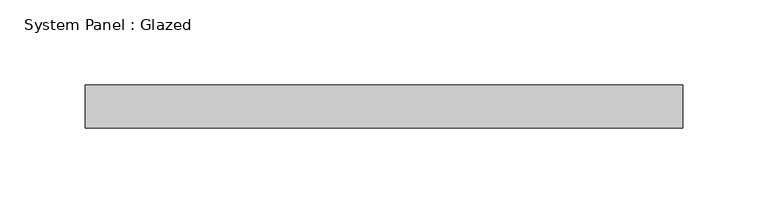
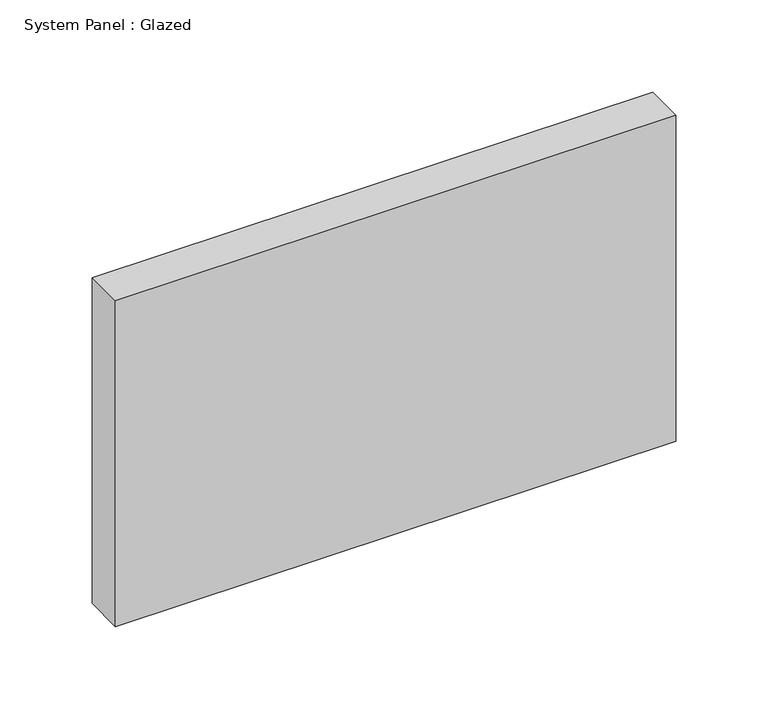
"""IFC4 building model written with IfcOpenShell, lengths in millimetres: plate geometry, System Panel : Glazed."""

from ifc_helpers import new_model, si_unit, origin, origin_with_axes, place, context, project, spatial, polyline, outline, extrude, source, transform, mapped, element, save


def system_panel_glazed_325805c1(model_context):
    return source(origin(), model_context, "Body", "SweptSolid", [
        extrude(outline(polyline([(175.6833333, 19.05), (-175.6833333, 19.05), (-175.6833333, 44.45), (175.6833333, 44.45), (175.6833333, 19.05)])), origin_with_axes(), (0.0, 0.0, 1.0), 215.9),
    ])


if __name__ == "__main__":
    model = new_model("IFC4")
    model_context = context("Model", 3, world=origin())
    ifc_project = project(units=[si_unit("LENGTHUNIT", "METRE", prefix="MILLI")], contexts=[model_context])
    site = spatial("IfcSite", under=ifc_project)
    building = spatial("IfcBuilding", under=site)
    placement = place(None, origin())
    system_panel_glazed_shape = system_panel_glazed_325805c1(model_context)
    element("IfcPlate", 1, ObjectType="System Panel : Glazed", at=placement, inside=building, context=model_context, shape_type="MappedRepresentation", body=[
        mapped(system_panel_glazed_shape, transform((0.0, 0.0, 0.0), x_axis=(1.0, 0.0, 0.0), y_axis=(0.0, 1.0, 0.0), z_axis=(0.0, 0.0, 1.0))),
    ])
    save(model, "model.ifc")

# Revit data of these elements
# Type "System Panel : Glazed"
#   Construction Type Id = "GSP4R"
#   Analytic Construction = "1/8 in Pilkington single glazing"
#   Visual Light Transmittance = 0.9
#   Solar Heat Gain Coefficient = 0.86
#   Heat Transfer Coefficient (U) = 1.18115 BTU/(h·ft²·°F)
#   Define Thermal Properties by = 1
# Element 1 (IfcPlate, "System Panel : Glazed")
#   Materials on its faces: "Glass"
# Materials
#   "Glass": class "Glass", colour RGB 0 128 192, transparency 0.75, Description = "Soda Lime Glass", Cost = 0
